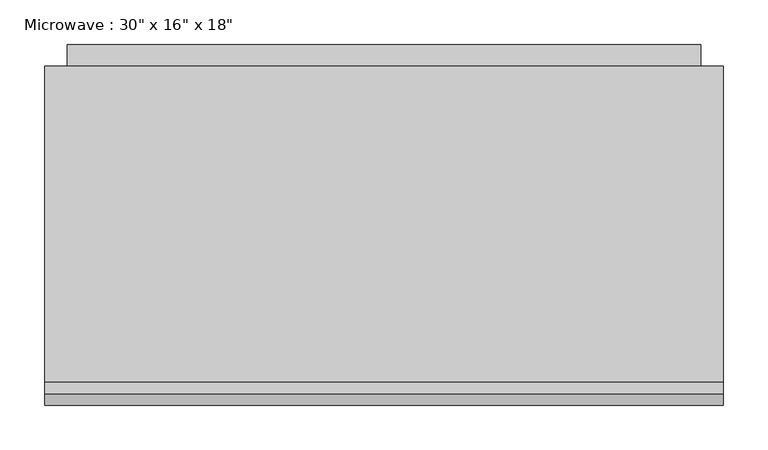
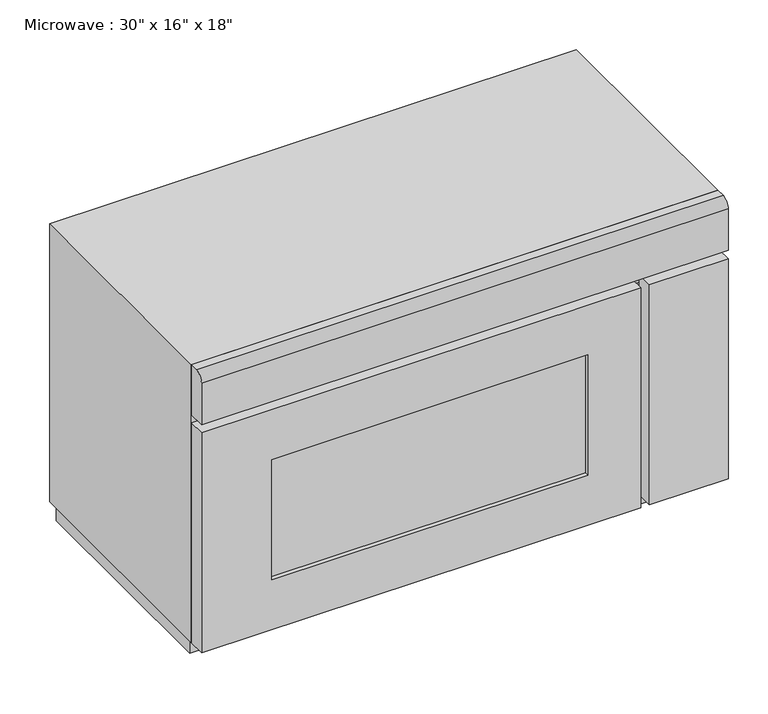
"""IFC4 building model written with IfcOpenShell, lengths in millimetres: proxy geometry."""

from ifc_helpers import new_model, si_unit, point, frame, frame_2d, origin, place, context, project, spatial, polyline, circle_curve, trimmed, segment, composite_curve, outline, extrude, faceted_brep, source, transform, mapped, element, save


def proxy_8a8d5ab2(model_context):
    return source(origin(), model_context, "Body", "SolidModel", [
        extrude(outline(polyline([(678.4897523, -549.9305058), (220.8928773, -549.9305058), (220.8928773, -543.5805058), (678.4897523, -543.5805058), (678.4897523, -549.9305058)])), frame((0.0, 0.0, 1022.35), z_axis=(0.0, 0.0, 1.0), x_axis=(1.0, 0.0, 0.0)), (0.0, 0.0, 1.0), 184.15),
        extrude(outline(polyline([(1282.7, 754.6897523), (1282.7, 119.2928773), (946.15, 119.2928773), (946.15, 754.6897523), (1282.7, 754.6897523)]), holes=[polyline([(1206.5, 678.4897523), (1022.35, 678.4897523), (1022.35, 220.8928773), (1206.5, 220.8928773), (1206.5, 678.4897523)])]), frame((0.0, -556.2805058, 0.0), z_axis=(0.0, 1.0, 0.0), x_axis=(0.0, 0.0, 1.0)), (0.0, 0.0, 1.0), 25.4),
        extrude(outline(polyline([(881.2928773, -556.2805058), (767.3897523, -556.2805058), (767.3897523, -530.8805058), (881.2928773, -530.8805058), (881.2928773, -556.2805058)])), frame((0.0, 0.0, 946.15), z_axis=(0.0, 0.0, 1.0), x_axis=(1.0, 0.0, 0.0)), (0.0, 0.0, 1.0), 336.55),
        extrude(outline(composite_curve([segment(polyline([(-543.5805058, 1371.6), (-530.8805058, 1371.6), (-530.8805058, 1295.4), (-556.2805058, 1295.4), (-556.2805058, 1358.9)]), True, "CONTINUOUS"), segment(trimmed(circle_curve(frame_2d((-543.5805058, 1358.9)), 12.7), [point((-556.2805058, 1358.9))], [point((-543.5805058, 1371.6))], False, "CARTESIAN"), True, "CONTINUOUS")], self_intersect=False)), frame((119.2928773, 0.0, 0.0), z_axis=(1.0, 0.0, 0.0), x_axis=(0.0, 1.0, 0.0)), (0.0, 0.0, 1.0), 762.0),
        extrude(outline(polyline([(-151.0441495, 1346.2), (-151.0441495, 961.946551), (-176.4441495, 936.546551), (-176.4441495, 1346.2), (-151.0441495, 1346.2)])), frame((144.6928773, 0.0, 0.0), z_axis=(1.0, 0.0, 0.0), x_axis=(0.0, 1.0, 0.0)), (0.0, 0.0, 1.0), 711.2),
        faceted_brep([(881.2928773, -175.2805058, 1371.6), (119.2928773, -175.2805058, 1371.6), (119.2928773, -530.8805058, 1371.6), (881.2928773, -530.8805058, 1371.6), (881.2928773, -175.2805058, 946.15), (881.2928773, -530.8805058, 946.15), (119.2928773, -530.8805058, 946.15), (119.2928773, -175.2805058, 946.15), (824.5397523, -530.8805058, 1271.0014904), (824.5397523, -530.8805058, 1020.1764904), (176.0460023, -530.8805058, 1020.1764904), (176.0460023, -530.8805058, 1271.0014904), (824.5397523, -200.6805058, 1271.0014904), (176.0460023, -200.6805058, 1271.0014904), (176.0460023, -200.6805058, 1020.1764904), (824.5397523, -200.6805058, 1020.1764904)], [[[0, 1, 2, 3]], [[4, 5, 6, 7]], [[1, 0, 4, 7]], [[2, 1, 7, 6]], [[3, 2, 6, 5], [8, 9, 10, 11]], [[0, 3, 5, 4]], [[12, 13, 14, 15]], [[12, 15, 9, 8]], [[15, 14, 10, 9]], [[14, 13, 11, 10]], [[13, 12, 8, 11]]]),
        extrude(outline(polyline([(871.7678773, -175.2805058), (871.7678773, -510.2430058), (128.8178773, -510.2430058), (128.8178773, -175.2805058), (871.7678773, -175.2805058)])), frame((0.0, 0.0, 914.4), z_axis=(0.0, 0.0, 1.0), x_axis=(1.0, 0.0, 0.0)), (0.0, 0.0, 1.0), 31.75),
    ])


if __name__ == "__main__":
    model = new_model("IFC4")
    model_context = context("Model", 3, world=origin())
    ifc_project = project(units=[si_unit("LENGTHUNIT", "METRE", prefix="MILLI")], contexts=[model_context])
    site = spatial("IfcSite", under=ifc_project)
    building = spatial("IfcBuilding", under=site)
    placement = place(None, origin())
    proxy_shape = proxy_8a8d5ab2(model_context)
    element("IfcBuildingElementProxy", 1, Name="Microwave : 30\" x 16\" x 18\"", ObjectType="Microwave : 30\" x 16\" x 18\"", at=placement, inside=building, context=model_context, shape_type="MappedRepresentation", body=[
        mapped(proxy_shape, transform((0.0, 0.0, 0.0), x_axis=(1.0, 0.0, 0.0), y_axis=(0.0, 1.0, 0.0), z_axis=(0.0, 0.0, 1.0))),
    ])
    save(model, "model.ifc")

# Revit data of these elements
# Type "Microwave : 30\" x 16\" x 18\""
#   Assembly Code = "E1090400"
#   Depth = 1' - 4"
#   Height = 1' - 6"
#   Width = 2' - 6"
#   Microwave Material = Laminate, Ivory, Matte
#   Default Elevation = 0
# Element 1 (IfcBuildingElementProxy, "Microwave : 30\" x 16\" x 18\"")
#   Materials on its faces: "Laminate, Ivory, Matte", "Glass"
# Materials
#   "Laminate, Ivory, Matte": class "Plastic", colour RGB 247 247 239, transparency 0, Description = "Plastic Laminate - Ivory, Matte", Cost = 0
#   "Glass": class "Glass", colour RGB 0 128 192, transparency 0.75, Description = "Soda Lime Glass", Cost = 0
